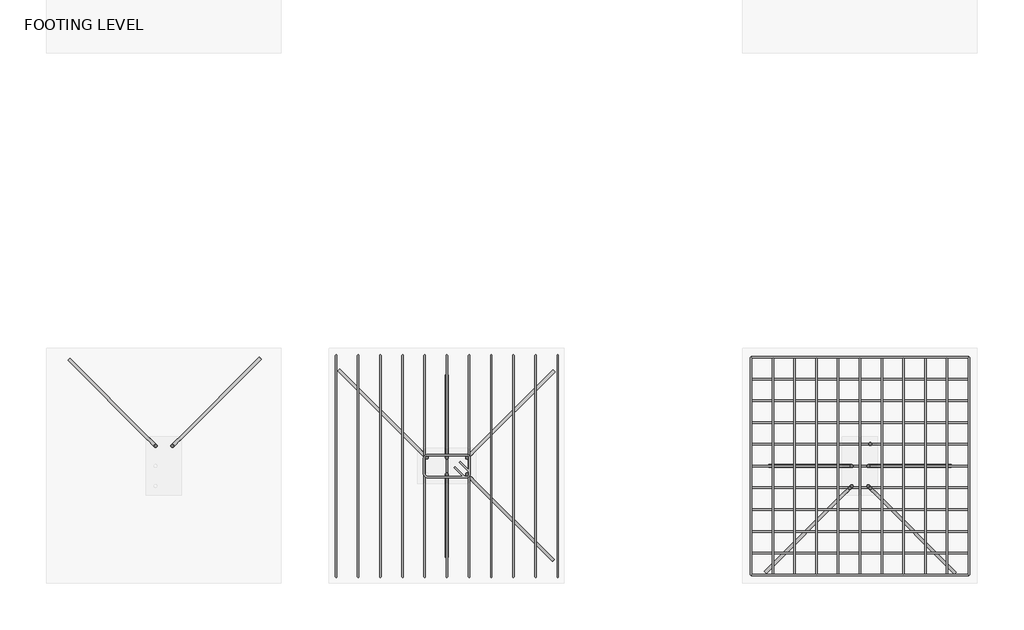
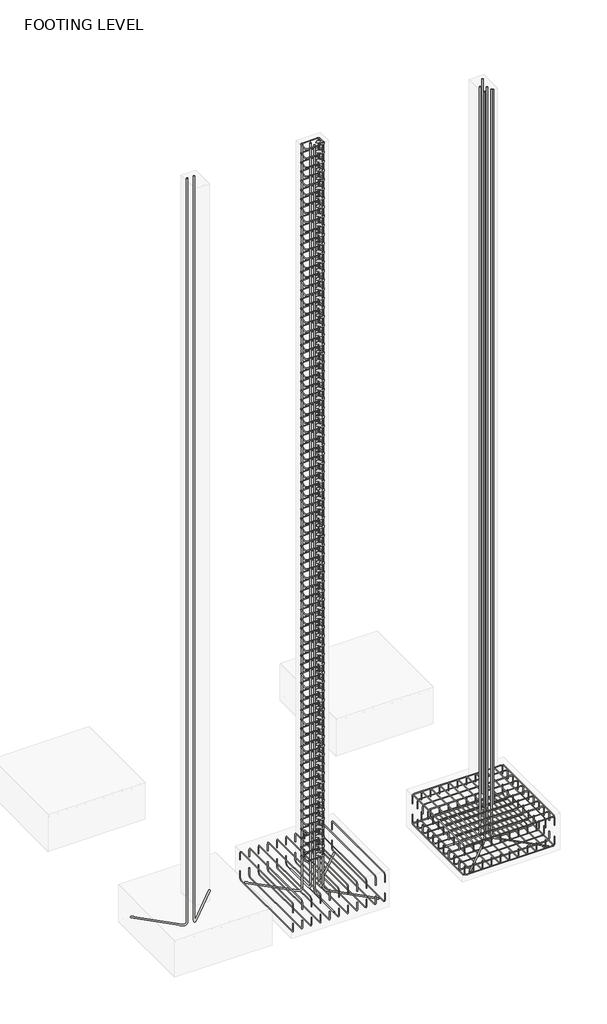
# One storey, part 8 of 10: 23 reinforcing bars.
"""IFC4 building model written with IfcOpenShell, lengths in millimetres."""

from ifc_helpers import new_model, si_unit, point, frame, origin, place, context, project, spatial, polyline, circle_curve, trimmed, segment, composite_curve, source, transform, mapped, element, save
from ifc_brep_helpers import swept_disk

model = new_model("IFC4")

# Units and contexts
model_context = context("Model", 3, world=origin())
ifc_project = project(units=[si_unit("LENGTHUNIT", "METRE", prefix="MILLI")], contexts=[model_context])

# Site, building, storey
site = spatial("IfcSite", under=ifc_project)
building = spatial("IfcBuilding", under=site)
storey = spatial("IfcBuildingStorey", under=building, Name="FOOTING LEVEL", Elevation=-1371.6)

# Reinforcing bars
placement = place(None, origin())
reinforcing_bar_shape = source(origin(), model_context, "Body", "SolidModel", [
    swept_disk(composite_curve([segment(polyline([(-9491.3043223, 10499.0953802, -1574.8), (-9491.3043223, 10499.0953802, -1460.5)]), True, "CONTINUOUS"), segment(trimmed(circle_curve(frame((-9491.3043223, 10465.7578802, -1460.5), z_axis=(1.0, 0.0, 0.0), x_axis=(0.0, 33.337499999999636, 0.0)), 33.3375), [point((-9491.3043223, 10499.0953802, -1460.5))], [point((-9491.3043223, 10465.7578802, -1427.1625))], True, "CARTESIAN"), True, "CONTINUOUS"), segment(polyline([(-9491.3043223, 10465.7578802, -1427.1625), (-9491.3043223, 9119.5578802, -1427.1625)]), True, "CONTINUOUS"), segment(trimmed(circle_curve(frame((-9491.3043223, 9119.5578802, -1460.5), z_axis=(1.0, 0.0, 0.0), x_axis=(0.0, 0.0, 33.33750000000009)), 33.3375), [point((-9491.3043223, 9119.5578802, -1427.1625))], [point((-9491.3043223, 9086.2203802, -1460.5))], True, "CARTESIAN"), True, "CONTINUOUS"), segment(polyline([(-9491.3043223, 9086.2203802, -1460.5), (-9491.3043223, 9086.2203802, -1574.8)]), True, "CONTINUOUS")], self_intersect=False), 4.7625),
])
element("IfcReinforcingBar", 1, at=placement, inside=storey, context=model_context, shape_type="MappedRepresentation", body=[
    mapped(reinforcing_bar_shape, transform((0.0, 0.0, 0.0), x_axis=(1.0, 0.0, 0.0), y_axis=(0.0, 1.0, 0.0), z_axis=(0.0, 0.0, 1.0))),
    mapped(reinforcing_bar_shape, transform((-141.2875, 0.0, 0.0), x_axis=(1.0, 0.0, 0.0), y_axis=(0.0, 1.0, 0.0), z_axis=(0.0, 0.0, 1.0))),
    mapped(reinforcing_bar_shape, transform((-282.575, 0.0, 0.0), x_axis=(1.0, 0.0, 0.0), y_axis=(0.0, 1.0, 0.0), z_axis=(0.0, 0.0, 1.0))),
    mapped(reinforcing_bar_shape, transform((-423.8625, 0.0, 0.0), x_axis=(1.0, 0.0, 0.0), y_axis=(0.0, 1.0, 0.0), z_axis=(0.0, 0.0, 1.0))),
    mapped(reinforcing_bar_shape, transform((-565.15, 0.0, 0.0), x_axis=(1.0, 0.0, 0.0), y_axis=(0.0, 1.0, 0.0), z_axis=(0.0, 0.0, 1.0))),
    mapped(reinforcing_bar_shape, transform((-706.4375, 0.0, 0.0), x_axis=(1.0, 0.0, 0.0), y_axis=(0.0, 1.0, 0.0), z_axis=(0.0, 0.0, 1.0))),
    mapped(reinforcing_bar_shape, transform((-847.725, 0.0, 0.0), x_axis=(1.0, 0.0, 0.0), y_axis=(0.0, 1.0, 0.0), z_axis=(0.0, 0.0, 1.0))),
    mapped(reinforcing_bar_shape, transform((-989.0125, 0.0, 0.0), x_axis=(1.0, 0.0, 0.0), y_axis=(0.0, 1.0, 0.0), z_axis=(0.0, 0.0, 1.0))),
    mapped(reinforcing_bar_shape, transform((-1130.3, 0.0, 0.0), x_axis=(1.0, 0.0, 0.0), y_axis=(0.0, 1.0, 0.0), z_axis=(0.0, 0.0, 1.0))),
    mapped(reinforcing_bar_shape, transform((-1271.5875, 0.0, 0.0), x_axis=(1.0, 0.0, 0.0), y_axis=(0.0, 1.0, 0.0), z_axis=(0.0, 0.0, 1.0))),
    mapped(reinforcing_bar_shape, transform((-1412.875, 0.0, 0.0), x_axis=(1.0, 0.0, 0.0), y_axis=(0.0, 1.0, 0.0), z_axis=(0.0, 0.0, 1.0))),
])
reinforcing_bar_2_shape = source(origin(), model_context, "Body", "SolidModel", [
    swept_disk(composite_curve([segment(polyline([(-9491.3043223, 9086.2203802, -1778.0), (-9491.3043223, 9086.2203802, -1892.3)]), True, "CONTINUOUS"), segment(trimmed(circle_curve(frame((-9491.3043223, 9119.5578802, -1892.3), z_axis=(1.0, 0.0, 0.0), x_axis=(0.0, -33.337499999999636, 0.0)), 33.3375), [point((-9491.3043223, 9086.2203802, -1892.3))], [point((-9491.3043223, 9119.5578802, -1925.6375))], True, "CARTESIAN"), True, "CONTINUOUS"), segment(polyline([(-9491.3043223, 9119.5578802, -1925.6375), (-9491.3043223, 10465.7578802, -1925.6375)]), True, "CONTINUOUS"), segment(trimmed(circle_curve(frame((-9491.3043223, 10465.7578802, -1892.3), z_axis=(1.0, 0.0, 0.0), x_axis=(0.0, 0.0, -33.33750000000009)), 33.3375), [point((-9491.3043223, 10465.7578802, -1925.6375))], [point((-9491.3043223, 10499.0953802, -1892.3))], True, "CARTESIAN"), True, "CONTINUOUS"), segment(polyline([(-9491.3043223, 10499.0953802, -1892.3), (-9491.3043223, 10499.0953802, -1778.0)]), True, "CONTINUOUS")], self_intersect=False), 4.7625),
])
element("IfcReinforcingBar", 2, at=placement, inside=storey, context=model_context, shape_type="MappedRepresentation", body=[
    mapped(reinforcing_bar_2_shape, transform((0.0, 0.0, 0.0), x_axis=(1.0, 0.0, 0.0), y_axis=(0.0, 1.0, 0.0), z_axis=(0.0, 0.0, 1.0))),
    mapped(reinforcing_bar_2_shape, transform((-141.2875, 0.0, 0.0), x_axis=(1.0, 0.0, 0.0), y_axis=(0.0, 1.0, 0.0), z_axis=(0.0, 0.0, 1.0))),
    mapped(reinforcing_bar_2_shape, transform((-282.575, 0.0, 0.0), x_axis=(1.0, 0.0, 0.0), y_axis=(0.0, 1.0, 0.0), z_axis=(0.0, 0.0, 1.0))),
    mapped(reinforcing_bar_2_shape, transform((-423.8625, 0.0, 0.0), x_axis=(1.0, 0.0, 0.0), y_axis=(0.0, 1.0, 0.0), z_axis=(0.0, 0.0, 1.0))),
    mapped(reinforcing_bar_2_shape, transform((-565.15, 0.0, 0.0), x_axis=(1.0, 0.0, 0.0), y_axis=(0.0, 1.0, 0.0), z_axis=(0.0, 0.0, 1.0))),
    mapped(reinforcing_bar_2_shape, transform((-706.4375, 0.0, 0.0), x_axis=(1.0, 0.0, 0.0), y_axis=(0.0, 1.0, 0.0), z_axis=(0.0, 0.0, 1.0))),
    mapped(reinforcing_bar_2_shape, transform((-847.725, 0.0, 0.0), x_axis=(1.0, 0.0, 0.0), y_axis=(0.0, 1.0, 0.0), z_axis=(0.0, 0.0, 1.0))),
    mapped(reinforcing_bar_2_shape, transform((-989.0125, 0.0, 0.0), x_axis=(1.0, 0.0, 0.0), y_axis=(0.0, 1.0, 0.0), z_axis=(0.0, 0.0, 1.0))),
    mapped(reinforcing_bar_2_shape, transform((-1130.3, 0.0, 0.0), x_axis=(1.0, 0.0, 0.0), y_axis=(0.0, 1.0, 0.0), z_axis=(0.0, 0.0, 1.0))),
    mapped(reinforcing_bar_2_shape, transform((-1271.5875, 0.0, 0.0), x_axis=(1.0, 0.0, 0.0), y_axis=(0.0, 1.0, 0.0), z_axis=(0.0, 0.0, 1.0))),
    mapped(reinforcing_bar_2_shape, transform((-1412.875, 0.0, 0.0), x_axis=(1.0, 0.0, 0.0), y_axis=(0.0, 1.0, 0.0), z_axis=(0.0, 0.0, 1.0))),
])
reinforcing_bar_3_shape = source(origin(), model_context, "Body", "SolidModel", [
    swept_disk(composite_curve([segment(polyline([(-10904.1793223, 9086.2203802, -1770.864029), (-10904.1793223, 9086.2203802, -1885.164029)]), True, "CONTINUOUS"), segment(trimmed(circle_curve(frame((-10870.8418223, 9086.2203802, -1885.164029), z_axis=(0.0, -1.0, 0.0), x_axis=(-33.337499999999636, 0.0, 0.0)), 33.3375), [point((-10904.1793223, 9086.2203802, -1885.164029))], [point((-10870.8418223, 9086.2203802, -1918.501529))], True, "CARTESIAN"), True, "CONTINUOUS"), segment(polyline([(-10870.8418223, 9086.2203802, -1918.501529), (-9524.6418223, 9086.2203802, -1918.501529)]), True, "CONTINUOUS"), segment(trimmed(circle_curve(frame((-9524.6418223, 9086.2203802, -1885.164029), z_axis=(0.0, -1.0, 0.0), x_axis=(0.0, 0.0, -33.337499999999864)), 33.3375), [point((-9524.6418223, 9086.2203802, -1918.501529))], [point((-9491.3043223, 9086.2203802, -1885.164029))], True, "CARTESIAN"), True, "CONTINUOUS"), segment(polyline([(-9491.3043223, 9086.2203802, -1885.164029), (-9491.3043223, 9086.2203802, -1770.864029)]), True, "CONTINUOUS")], self_intersect=False), 4.7625),
])
element("IfcReinforcingBar", 3, at=placement, inside=storey, context=model_context, shape_type="MappedRepresentation", body=[
    mapped(reinforcing_bar_3_shape, transform((0.0, 0.0, 0.0), x_axis=(1.0, 0.0, 0.0), y_axis=(0.0, 1.0, 0.0), z_axis=(0.0, 0.0, 1.0))),
    mapped(reinforcing_bar_3_shape, transform((0.0, 141.2875, 0.0), x_axis=(1.0, 0.0, 0.0), y_axis=(0.0, 1.0, 0.0), z_axis=(0.0, 0.0, 1.0))),
    mapped(reinforcing_bar_3_shape, transform((0.0, 282.575, 0.0), x_axis=(1.0, 0.0, 0.0), y_axis=(0.0, 1.0, 0.0), z_axis=(0.0, 0.0, 1.0))),
    mapped(reinforcing_bar_3_shape, transform((0.0, 423.8625, 0.0), x_axis=(1.0, 0.0, 0.0), y_axis=(0.0, 1.0, 0.0), z_axis=(0.0, 0.0, 1.0))),
    mapped(reinforcing_bar_3_shape, transform((0.0, 565.15, 0.0), x_axis=(1.0, 0.0, 0.0), y_axis=(0.0, 1.0, 0.0), z_axis=(0.0, 0.0, 1.0))),
    mapped(reinforcing_bar_3_shape, transform((0.0, 706.4375, 0.0), x_axis=(1.0, 0.0, 0.0), y_axis=(0.0, 1.0, 0.0), z_axis=(0.0, 0.0, 1.0))),
    mapped(reinforcing_bar_3_shape, transform((0.0, 847.725, 0.0), x_axis=(1.0, 0.0, 0.0), y_axis=(0.0, 1.0, 0.0), z_axis=(0.0, 0.0, 1.0))),
    mapped(reinforcing_bar_3_shape, transform((0.0, 989.0125, 0.0), x_axis=(1.0, 0.0, 0.0), y_axis=(0.0, 1.0, 0.0), z_axis=(0.0, 0.0, 1.0))),
    mapped(reinforcing_bar_3_shape, transform((0.0, 1130.3, 0.0), x_axis=(1.0, 0.0, 0.0), y_axis=(0.0, 1.0, 0.0), z_axis=(0.0, 0.0, 1.0))),
    mapped(reinforcing_bar_3_shape, transform((0.0, 1271.5875, 0.0), x_axis=(1.0, 0.0, 0.0), y_axis=(0.0, 1.0, 0.0), z_axis=(0.0, 0.0, 1.0))),
    mapped(reinforcing_bar_3_shape, transform((0.0, 1412.875, 0.0), x_axis=(1.0, 0.0, 0.0), y_axis=(0.0, 1.0, 0.0), z_axis=(0.0, 0.0, 1.0))),
])
reinforcing_bar_4_shape = source(origin(), model_context, "Body", "SolidModel", [
    swept_disk(composite_curve([segment(polyline([(-10904.1793223, 10499.0953802, -1586.5406765), (-10904.1793223, 10499.0953802, -1472.2406765)]), True, "CONTINUOUS"), segment(trimmed(circle_curve(frame((-10870.8418223, 10499.0953802, -1472.2406765), z_axis=(0.0, 1.0, 0.0), x_axis=(-33.337499999999636, 0.0, 0.0)), 33.3375), [point((-10904.1793223, 10499.0953802, -1472.2406765))], [point((-10870.8418223, 10499.0953802, -1438.9031765))], True, "CARTESIAN"), True, "CONTINUOUS"), segment(polyline([(-10870.8418223, 10499.0953802, -1438.9031765), (-9524.6418223, 10499.0953802, -1438.9031765)]), True, "CONTINUOUS"), segment(trimmed(circle_curve(frame((-9524.6418223, 10499.0953802, -1472.2406765), z_axis=(0.0, 1.0, 0.0), x_axis=(0.0, 0.0, 33.33750000000009)), 33.3375), [point((-9524.6418223, 10499.0953802, -1438.9031765))], [point((-9491.3043223, 10499.0953802, -1472.2406765))], True, "CARTESIAN"), True, "CONTINUOUS"), segment(polyline([(-9491.3043223, 10499.0953802, -1472.2406765), (-9491.3043223, 10499.0953802, -1586.5406765)]), True, "CONTINUOUS")], self_intersect=False), 4.7625),
])
element("IfcReinforcingBar", 4, at=placement, inside=storey, context=model_context, shape_type="MappedRepresentation", body=[
    mapped(reinforcing_bar_4_shape, transform((0.0, 0.0, 0.0), x_axis=(1.0, 0.0, 0.0), y_axis=(0.0, 1.0, 0.0), z_axis=(0.0, 0.0, 1.0))),
    mapped(reinforcing_bar_4_shape, transform((0.0, -141.2875, 0.0), x_axis=(1.0, 0.0, 0.0), y_axis=(0.0, 1.0, 0.0), z_axis=(0.0, 0.0, 1.0))),
    mapped(reinforcing_bar_4_shape, transform((0.0, -282.575, 0.0), x_axis=(1.0, 0.0, 0.0), y_axis=(0.0, 1.0, 0.0), z_axis=(0.0, 0.0, 1.0))),
    mapped(reinforcing_bar_4_shape, transform((0.0, -423.8625, 0.0), x_axis=(1.0, 0.0, 0.0), y_axis=(0.0, 1.0, 0.0), z_axis=(0.0, 0.0, 1.0))),
    mapped(reinforcing_bar_4_shape, transform((0.0, -565.15, 0.0), x_axis=(1.0, 0.0, 0.0), y_axis=(0.0, 1.0, 0.0), z_axis=(0.0, 0.0, 1.0))),
    mapped(reinforcing_bar_4_shape, transform((0.0, -706.4375, 0.0), x_axis=(1.0, 0.0, 0.0), y_axis=(0.0, 1.0, 0.0), z_axis=(0.0, 0.0, 1.0))),
    mapped(reinforcing_bar_4_shape, transform((0.0, -847.725, 0.0), x_axis=(1.0, 0.0, 0.0), y_axis=(0.0, 1.0, 0.0), z_axis=(0.0, 0.0, 1.0))),
    mapped(reinforcing_bar_4_shape, transform((0.0, -989.0125, 0.0), x_axis=(1.0, 0.0, 0.0), y_axis=(0.0, 1.0, 0.0), z_axis=(0.0, 0.0, 1.0))),
    mapped(reinforcing_bar_4_shape, transform((0.0, -1130.3, 0.0), x_axis=(1.0, 0.0, 0.0), y_axis=(0.0, 1.0, 0.0), z_axis=(0.0, 0.0, 1.0))),
    mapped(reinforcing_bar_4_shape, transform((0.0, -1271.5875, 0.0), x_axis=(1.0, 0.0, 0.0), y_axis=(0.0, 1.0, 0.0), z_axis=(0.0, 0.0, 1.0))),
    mapped(reinforcing_bar_4_shape, transform((0.0, -1412.875, 0.0), x_axis=(1.0, 0.0, 0.0), y_axis=(0.0, 1.0, 0.0), z_axis=(0.0, 0.0, 1.0))),
])
reinforcing_bar_5_shape = source(origin(), model_context, "Body", "SolidModel", [
    swept_disk(composite_curve([segment(polyline([(-12158.3043223, 9073.5203802, -1770.864029), (-12158.3043223, 9073.5203802, -1885.164029)]), True, "CONTINUOUS"), segment(trimmed(circle_curve(frame((-12158.3043223, 9106.8578802, -1885.164029), z_axis=(1.0, 0.0, 0.0), x_axis=(0.0, -33.337499999999636, 0.0)), 33.3375), [point((-12158.3043223, 9073.5203802, -1885.164029))], [point((-12158.3043223, 9106.8578802, -1918.501529))], True, "CARTESIAN"), True, "CONTINUOUS"), segment(polyline([(-12158.3043223, 9106.8578802, -1918.501529), (-12158.3043223, 10478.4578802, -1918.501529)]), True, "CONTINUOUS"), segment(trimmed(circle_curve(frame((-12158.3043223, 10478.4578802, -1885.164029), z_axis=(1.0, 0.0, 0.0), x_axis=(0.0, 0.0, -33.337499999999864)), 33.3375), [point((-12158.3043223, 10478.4578802, -1918.501529))], [point((-12158.3043223, 10511.7953802, -1885.164029))], True, "CARTESIAN"), True, "CONTINUOUS"), segment(polyline([(-12158.3043223, 10511.7953802, -1885.164029), (-12158.3043223, 10511.7953802, -1770.864029)]), True, "CONTINUOUS")], self_intersect=False), 4.7625),
])
element("IfcReinforcingBar", 5, at=placement, inside=storey, context=model_context, shape_type="MappedRepresentation", body=[
    mapped(reinforcing_bar_5_shape, transform((0.0, 0.0, 0.0), x_axis=(1.0, 0.0, 0.0), y_axis=(0.0, 1.0, 0.0), z_axis=(0.0, 0.0, 1.0))),
    mapped(reinforcing_bar_5_shape, transform((-143.8275, 0.0, 0.0), x_axis=(1.0, 0.0, 0.0), y_axis=(0.0, 1.0, 0.0), z_axis=(0.0, 0.0, 1.0))),
    mapped(reinforcing_bar_5_shape, transform((-287.655, 0.0, 0.0), x_axis=(1.0, 0.0, 0.0), y_axis=(0.0, 1.0, 0.0), z_axis=(0.0, 0.0, 1.0))),
    mapped(reinforcing_bar_5_shape, transform((-431.4825, 0.0, 0.0), x_axis=(1.0, 0.0, 0.0), y_axis=(0.0, 1.0, 0.0), z_axis=(0.0, 0.0, 1.0))),
    mapped(reinforcing_bar_5_shape, transform((-575.31, 0.0, 0.0), x_axis=(1.0, 0.0, 0.0), y_axis=(0.0, 1.0, 0.0), z_axis=(0.0, 0.0, 1.0))),
    mapped(reinforcing_bar_5_shape, transform((-719.1375, 0.0, 0.0), x_axis=(1.0, 0.0, 0.0), y_axis=(0.0, 1.0, 0.0), z_axis=(0.0, 0.0, 1.0))),
    mapped(reinforcing_bar_5_shape, transform((-862.965, 0.0, 0.0), x_axis=(1.0, 0.0, 0.0), y_axis=(0.0, 1.0, 0.0), z_axis=(0.0, 0.0, 1.0))),
    mapped(reinforcing_bar_5_shape, transform((-1006.7925, 0.0, 0.0), x_axis=(1.0, 0.0, 0.0), y_axis=(0.0, 1.0, 0.0), z_axis=(0.0, 0.0, 1.0))),
    mapped(reinforcing_bar_5_shape, transform((-1150.62, 0.0, 0.0), x_axis=(1.0, 0.0, 0.0), y_axis=(0.0, 1.0, 0.0), z_axis=(0.0, 0.0, 1.0))),
    mapped(reinforcing_bar_5_shape, transform((-1294.4475, 0.0, 0.0), x_axis=(1.0, 0.0, 0.0), y_axis=(0.0, 1.0, 0.0), z_axis=(0.0, 0.0, 1.0))),
    mapped(reinforcing_bar_5_shape, transform((-1438.275, 0.0, 0.0), x_axis=(1.0, 0.0, 0.0), y_axis=(0.0, 1.0, 0.0), z_axis=(0.0, 0.0, 1.0))),
])
reinforcing_bar_6_shape = source(origin(), model_context, "Body", "SolidModel", [
    swept_disk(composite_curve([segment(polyline([(-13596.5793223, 9073.5203802, -1586.5406765), (-13596.5793223, 9073.5203802, -1472.2406765)]), True, "CONTINUOUS"), segment(trimmed(circle_curve(frame((-13596.5793223, 9106.8578802, -1472.2406765), z_axis=(-1.0, 0.0, 0.0), x_axis=(0.0, -33.337499999999636, 0.0)), 33.3375), [point((-13596.5793223, 9073.5203802, -1472.2406765))], [point((-13596.5793223, 9106.8578802, -1438.9031765))], True, "CARTESIAN"), True, "CONTINUOUS"), segment(polyline([(-13596.5793223, 9106.8578802, -1438.9031765), (-13596.5793223, 10478.4578802, -1438.9031765)]), True, "CONTINUOUS"), segment(trimmed(circle_curve(frame((-13596.5793223, 10478.4578802, -1472.2406765), z_axis=(-1.0, 0.0, 0.0), x_axis=(0.0, 0.0, 33.33750000000009)), 33.3375), [point((-13596.5793223, 10478.4578802, -1438.9031765))], [point((-13596.5793223, 10511.7953802, -1472.2406765))], True, "CARTESIAN"), True, "CONTINUOUS"), segment(polyline([(-13596.5793223, 10511.7953802, -1472.2406765), (-13596.5793223, 10511.7953802, -1586.5406765)]), True, "CONTINUOUS")], self_intersect=False), 4.7625),
])
element("IfcReinforcingBar", 6, at=placement, inside=storey, context=model_context, shape_type="MappedRepresentation", body=[
    mapped(reinforcing_bar_6_shape, transform((0.0, 0.0, 0.0), x_axis=(1.0, 0.0, 0.0), y_axis=(0.0, 1.0, 0.0), z_axis=(0.0, 0.0, 1.0))),
    mapped(reinforcing_bar_6_shape, transform((143.8275, 0.0, 0.0), x_axis=(1.0, 0.0, 0.0), y_axis=(0.0, 1.0, 0.0), z_axis=(0.0, 0.0, 1.0))),
    mapped(reinforcing_bar_6_shape, transform((287.655, 0.0, 0.0), x_axis=(1.0, 0.0, 0.0), y_axis=(0.0, 1.0, 0.0), z_axis=(0.0, 0.0, 1.0))),
    mapped(reinforcing_bar_6_shape, transform((431.4825, 0.0, 0.0), x_axis=(1.0, 0.0, 0.0), y_axis=(0.0, 1.0, 0.0), z_axis=(0.0, 0.0, 1.0))),
    mapped(reinforcing_bar_6_shape, transform((575.31, 0.0, 0.0), x_axis=(1.0, 0.0, 0.0), y_axis=(0.0, 1.0, 0.0), z_axis=(0.0, 0.0, 1.0))),
    mapped(reinforcing_bar_6_shape, transform((719.1375, 0.0, 0.0), x_axis=(1.0, 0.0, 0.0), y_axis=(0.0, 1.0, 0.0), z_axis=(0.0, 0.0, 1.0))),
    mapped(reinforcing_bar_6_shape, transform((862.965, 0.0, 0.0), x_axis=(1.0, 0.0, 0.0), y_axis=(0.0, 1.0, 0.0), z_axis=(0.0, 0.0, 1.0))),
    mapped(reinforcing_bar_6_shape, transform((1006.7925, 0.0, 0.0), x_axis=(1.0, 0.0, 0.0), y_axis=(0.0, 1.0, 0.0), z_axis=(0.0, 0.0, 1.0))),
    mapped(reinforcing_bar_6_shape, transform((1150.62, 0.0, 0.0), x_axis=(1.0, 0.0, 0.0), y_axis=(0.0, 1.0, 0.0), z_axis=(0.0, 0.0, 1.0))),
    mapped(reinforcing_bar_6_shape, transform((1294.4475, 0.0, 0.0), x_axis=(1.0, 0.0, 0.0), y_axis=(0.0, 1.0, 0.0), z_axis=(0.0, 0.0, 1.0))),
    mapped(reinforcing_bar_6_shape, transform((1438.275, 0.0, 0.0), x_axis=(1.0, 0.0, 0.0), y_axis=(0.0, 1.0, 0.0), z_axis=(0.0, 0.0, 1.0))),
])
element("IfcReinforcingBar", 7, at=placement, inside=storey, context=model_context, shape_type="SolidModel", body=[
    swept_disk(composite_curve([segment(polyline([(-15328.6277703, 10484.8938282, -1910.4342608), (-14814.0983591, 9970.3644169, -1910.4342608)]), True, "CONTINUOUS"), segment(trimmed(circle_curve(frame((-14814.0983591, 9970.3644169, -1843.7592608), z_axis=(-0.7071067811865736, -0.7071067811865216, 0.0), x_axis=(0.0, 0.0, -66.67499999999995)), 66.675), [point((-14814.0983591, 9970.3644169, -1910.4342608))], [point((-14766.9520144, 9923.2180723, -1843.7592608))], True, "CARTESIAN"), True, "CONTINUOUS"), segment(polyline([(-14766.9520144, 9923.2180723, -1843.7592608), (-14766.9520144, 9923.2180723, 10477.5)]), True, "CONTINUOUS")], self_intersect=False), 9.525),
])
element("IfcReinforcingBar", 8, at=placement, inside=storey, context=model_context, shape_type="SolidModel", body=[
    swept_disk(composite_curve([segment(polyline([(-14088.5374965, 10492.912206, -1910.4342608), (-14611.0852856, 9970.3644169, -1910.4342608)]), True, "CONTINUOUS"), segment(trimmed(circle_curve(frame((-14611.0852856, 9970.3644169, -1843.7592608), z_axis=(-0.7071067811865712, 0.7071067811865238, 0.0), x_axis=(0.0, 0.0, -66.67499999999995)), 66.675), [point((-14611.0852856, 9970.3644169, -1910.4342608))], [point((-14658.2316302, 9923.2180723, -1843.7592608))], True, "CARTESIAN"), True, "CONTINUOUS"), segment(polyline([(-14658.2316302, 9923.2180723, -1843.7592608), (-14658.2316302, 9923.2180723, 10477.5)]), True, "CONTINUOUS")], self_intersect=False), 9.525),
])
element("IfcReinforcingBar", 9, at=placement, inside=storey, context=model_context, shape_type="SolidModel", body=[
    swept_disk(composite_curve([segment(polyline([(-10130.6816302, 9935.9180723, -1346.2), (-10130.6816302, 9935.9180723, 10490.2)]), True, "CONTINUOUS")], self_intersect=False), 9.525),
])
element("IfcReinforcingBar", 10, at=placement, inside=storey, context=model_context, shape_type="SolidModel", body=[
    swept_disk(composite_curve([segment(polyline([(-10264.8020144, 9649.3976881, -1346.2), (-10264.8020144, 9649.3976881, 10490.2)]), True, "CONTINUOUS")], self_intersect=False), 9.525),
])
element("IfcReinforcingBar", 11, at=placement, inside=storey, context=model_context, shape_type="SolidModel", body=[
    swept_disk(composite_curve([segment(polyline([(-10130.6816302, 9649.3976881, -1346.2), (-10130.6816302, 9649.3976881, 10490.2)]), True, "CONTINUOUS")], self_intersect=False), 9.525),
])
element("IfcReinforcingBar", 12, at=placement, inside=storey, context=model_context, shape_type="SolidModel", body=[
    swept_disk(composite_curve([segment(polyline([(-10810.8211349, 9103.3785676, -1910.4342608), (-10299.2483591, 9614.9513434, -1910.4342608)]), True, "CONTINUOUS"), segment(trimmed(circle_curve(frame((-10299.2483591, 9614.9513434, -1843.7592608), z_axis=(0.7071067811865759, -0.7071067811865193, 0.0), x_axis=(0.0, 0.0, -66.67499999999995)), 66.675), [point((-10299.2483591, 9614.9513434, -1910.4342608))], [point((-10252.1020144, 9662.0976881, -1843.7592608))], True, "CARTESIAN"), True, "CONTINUOUS"), segment(polyline([(-10252.1020144, 9662.0976881, -1843.7592608), (-10252.1020144, 9662.0976881, 10490.2)]), True, "CONTINUOUS")], self_intersect=False), 9.525),
])
element("IfcReinforcingBar", 13, at=placement, inside=storey, context=model_context, shape_type="SolidModel", body=[
    swept_disk(composite_curve([segment(polyline([(-9579.2028099, 9097.9188678, -1910.4342608), (-10096.2352856, 9614.9513434, -1910.4342608)]), True, "CONTINUOUS"), segment(trimmed(circle_curve(frame((-10096.2352856, 9614.9513434, -1843.7592608), z_axis=(0.707106781186569, 0.707106781186526, 0.0), x_axis=(0.0, 0.0, -66.67499999999995)), 66.675), [point((-10096.2352856, 9614.9513434, -1910.4342608))], [point((-10143.3816302, 9662.0976881, -1843.7592608))], True, "CARTESIAN"), True, "CONTINUOUS"), segment(polyline([(-10143.3816302, 9662.0976881, -1843.7592608), (-10143.3816302, 9662.0976881, 10490.2)]), True, "CONTINUOUS")], self_intersect=False), 9.525),
])
element("IfcReinforcingBar", 14, at=placement, inside=storey, context=model_context, shape_type="SolidModel", body=[
    swept_disk(composite_curve([segment(polyline([(-10790.3318909, 9792.6578802, -1910.4342608), (-10318.7770144, 9792.6578802, -1910.4342608)]), True, "CONTINUOUS"), segment(trimmed(circle_curve(frame((-10318.7770144, 9792.6578802, -1843.7592608), z_axis=(0.0, -1.0, 0.0), x_axis=(0.0, 0.0, -66.67499999999995)), 66.675), [point((-10318.7770144, 9792.6578802, -1910.4342608))], [point((-10252.1020144, 9792.6578802, -1843.7592608))], True, "CARTESIAN"), True, "CONTINUOUS"), segment(polyline([(-10252.1020144, 9792.6578802, -1843.7592608), (-10252.1020144, 9792.6578802, 10490.2)]), True, "CONTINUOUS")], self_intersect=False), 9.525),
])
element("IfcReinforcingBar", 15, at=placement, inside=storey, context=model_context, shape_type="SolidModel", body=[
    swept_disk(composite_curve([segment(polyline([(-9605.1517538, 9792.6578802, -1916.7848067), (-10076.7066302, 9792.6578802, -1916.7848067)]), True, "CONTINUOUS"), segment(trimmed(circle_curve(frame((-10076.7066302, 9792.6578802, -1850.1098067), z_axis=(0.0, 1.0, 0.0), x_axis=(0.0, 0.0, -66.67499999999995)), 66.675), [point((-10076.7066302, 9792.6578802, -1916.7848067))], [point((-10143.3816302, 9792.6578802, -1850.1098067))], True, "CARTESIAN"), True, "CONTINUOUS"), segment(polyline([(-10143.3816302, 9792.6578802, -1850.1098067), (-10143.3816302, 9792.6578802, 10449.7223493)]), True, "CONTINUOUS")], self_intersect=False), 9.525),
])
reinforcing_bar_7_shape = source(origin(), model_context, "Body", "SolidModel", [
    swept_disk(composite_curve([segment(polyline([(-12827.3189996, 9785.059097, -1328.7375), (-12770.4548026, 9728.1948999, -1328.7375)]), True, "CONTINUOUS"), segment(trimmed(circle_curve(frame((-12753.6168223, 9745.0328802, -1328.7375), z_axis=(0.0, 0.0, 1.0), x_axis=(-16.83798029999889, -16.83798030000071, 0.0)), 23.8125), [point((-12770.4548026, 9728.1948999, -1328.7375))], [point((-12729.8043223, 9745.0328802, -1328.7375))], True, "CARTESIAN"), True, "CONTINUOUS"), segment(polyline([(-12729.8043223, 9745.0328802, -1328.7375), (-12729.8043223, 9840.2828802, -1328.7375)]), True, "CONTINUOUS"), segment(trimmed(circle_curve(frame((-12753.6168223, 9840.2828802, -1328.7375), z_axis=(0.0, 0.0, 1.0), x_axis=(23.8125, 0.0, 0.0)), 23.8125), [point((-12729.8043223, 9840.2828802, -1328.7375))], [point((-12753.6168223, 9864.0953802, -1328.7375))], True, "CARTESIAN"), True, "CONTINUOUS"), segment(polyline([(-12753.6168223, 9864.0953802, -1328.7375), (-13001.2668223, 9864.0953802, -1328.7375)]), True, "CONTINUOUS"), segment(trimmed(circle_curve(frame((-13001.2668223, 9840.3356211, -1330.3214839), z_axis=(0.0, -0.06651901052377396, 0.9977851578566089), x_axis=(0.0, 23.759759100001247, 1.583983900000021)), 23.8125), [point((-13001.2668223, 9864.0953802, -1328.7375))], [point((-13025.0793223, 9840.3356211, -1330.3214839))], True, "CARTESIAN"), True, "CONTINUOUS"), segment(polyline([(-13025.0793223, 9840.3356211, -1330.3214839), (-13025.0793223, 9744.9801392, -1336.6785161)]), True, "CONTINUOUS"), segment(trimmed(circle_curve(frame((-13001.2668223, 9744.9801392, -1336.6785161), z_axis=(0.0, -0.06651901052377396, 0.9977851578566089), x_axis=(-23.8125, 0.0, 0.0)), 23.8125), [point((-13025.0793223, 9744.9801392, -1336.6785161))], [point((-13001.2668223, 9721.2203802, -1338.2625))], True, "CARTESIAN"), True, "CONTINUOUS"), segment(polyline([(-13001.2668223, 9721.2203802, -1338.2625), (-12753.6168223, 9721.2203802, -1338.2625)]), True, "CONTINUOUS"), segment(trimmed(circle_curve(frame((-12753.6168223, 9745.0328802, -1338.2625), z_axis=(0.0, 0.0, 1.0), x_axis=(0.0, -23.8125, 0.0)), 23.8125), [point((-12753.6168223, 9721.2203802, -1338.2625))], [point((-12736.7788421, 9761.8708604, -1338.2625))], True, "CARTESIAN"), True, "CONTINUOUS"), segment(polyline([(-12736.7788421, 9761.8708604, -1338.2625), (-12793.6430392, 9818.7350575, -1338.2625)]), True, "CONTINUOUS")], self_intersect=False), 4.7625),
])
element("IfcReinforcingBar", 16, at=placement, inside=storey, context=model_context, shape_type="MappedRepresentation", body=[
    mapped(reinforcing_bar_7_shape, transform((0.0, 0.0, 0.0), x_axis=(1.0, 0.0, 0.0), y_axis=(0.0, 1.0, 0.0), z_axis=(0.0, 0.0, 1.0))),
    mapped(reinforcing_bar_7_shape, transform((0.0, 0.0, 151.3009615), x_axis=(1.0, 0.0, 0.0), y_axis=(0.0, 1.0, 0.0), z_axis=(0.0, 0.0, 1.0))),
    mapped(reinforcing_bar_7_shape, transform((0.0, 0.0, 302.6019231), x_axis=(1.0, 0.0, 0.0), y_axis=(0.0, 1.0, 0.0), z_axis=(0.0, 0.0, 1.0))),
    mapped(reinforcing_bar_7_shape, transform((0.0, 0.0, 453.9028846), x_axis=(1.0, 0.0, 0.0), y_axis=(0.0, 1.0, 0.0), z_axis=(0.0, 0.0, 1.0))),
    mapped(reinforcing_bar_7_shape, transform((0.0, 0.0, 605.2038462), x_axis=(1.0, 0.0, 0.0), y_axis=(0.0, 1.0, 0.0), z_axis=(0.0, 0.0, 1.0))),
    mapped(reinforcing_bar_7_shape, transform((0.0, 0.0, 756.5048077), x_axis=(1.0, 0.0, 0.0), y_axis=(0.0, 1.0, 0.0), z_axis=(0.0, 0.0, 1.0))),
    mapped(reinforcing_bar_7_shape, transform((0.0, 0.0, 907.8057692), x_axis=(1.0, 0.0, 0.0), y_axis=(0.0, 1.0, 0.0), z_axis=(0.0, 0.0, 1.0))),
    mapped(reinforcing_bar_7_shape, transform((0.0, 0.0, 1059.1067308), x_axis=(1.0, 0.0, 0.0), y_axis=(0.0, 1.0, 0.0), z_axis=(0.0, 0.0, 1.0))),
    mapped(reinforcing_bar_7_shape, transform((0.0, 0.0, 1210.4076923), x_axis=(1.0, 0.0, 0.0), y_axis=(0.0, 1.0, 0.0), z_axis=(0.0, 0.0, 1.0))),
    mapped(reinforcing_bar_7_shape, transform((0.0, 0.0, 1361.7086538), x_axis=(1.0, 0.0, 0.0), y_axis=(0.0, 1.0, 0.0), z_axis=(0.0, 0.0, 1.0))),
    mapped(reinforcing_bar_7_shape, transform((0.0, 0.0, 1513.0096154), x_axis=(1.0, 0.0, 0.0), y_axis=(0.0, 1.0, 0.0), z_axis=(0.0, 0.0, 1.0))),
    mapped(reinforcing_bar_7_shape, transform((0.0, 0.0, 1664.3105769), x_axis=(1.0, 0.0, 0.0), y_axis=(0.0, 1.0, 0.0), z_axis=(0.0, 0.0, 1.0))),
    mapped(reinforcing_bar_7_shape, transform((0.0, 0.0, 1815.6115385), x_axis=(1.0, 0.0, 0.0), y_axis=(0.0, 1.0, 0.0), z_axis=(0.0, 0.0, 1.0))),
    mapped(reinforcing_bar_7_shape, transform((0.0, 0.0, 1966.9125), x_axis=(1.0, 0.0, 0.0), y_axis=(0.0, 1.0, 0.0), z_axis=(0.0, 0.0, 1.0))),
    mapped(reinforcing_bar_7_shape, transform((0.0, 0.0, 2118.2134615), x_axis=(1.0, 0.0, 0.0), y_axis=(0.0, 1.0, 0.0), z_axis=(0.0, 0.0, 1.0))),
    mapped(reinforcing_bar_7_shape, transform((0.0, 0.0, 2269.5144231), x_axis=(1.0, 0.0, 0.0), y_axis=(0.0, 1.0, 0.0), z_axis=(0.0, 0.0, 1.0))),
    mapped(reinforcing_bar_7_shape, transform((0.0, 0.0, 2420.8153846), x_axis=(1.0, 0.0, 0.0), y_axis=(0.0, 1.0, 0.0), z_axis=(0.0, 0.0, 1.0))),
    mapped(reinforcing_bar_7_shape, transform((0.0, 0.0, 2572.1163462), x_axis=(1.0, 0.0, 0.0), y_axis=(0.0, 1.0, 0.0), z_axis=(0.0, 0.0, 1.0))),
    mapped(reinforcing_bar_7_shape, transform((0.0, 0.0, 2723.4173077), x_axis=(1.0, 0.0, 0.0), y_axis=(0.0, 1.0, 0.0), z_axis=(0.0, 0.0, 1.0))),
    mapped(reinforcing_bar_7_shape, transform((0.0, 0.0, 2874.7182692), x_axis=(1.0, 0.0, 0.0), y_axis=(0.0, 1.0, 0.0), z_axis=(0.0, 0.0, 1.0))),
    mapped(reinforcing_bar_7_shape, transform((0.0, 0.0, 3026.0192308), x_axis=(1.0, 0.0, 0.0), y_axis=(0.0, 1.0, 0.0), z_axis=(0.0, 0.0, 1.0))),
    mapped(reinforcing_bar_7_shape, transform((0.0, 0.0, 3177.3201923), x_axis=(1.0, 0.0, 0.0), y_axis=(0.0, 1.0, 0.0), z_axis=(0.0, 0.0, 1.0))),
    mapped(reinforcing_bar_7_shape, transform((0.0, 0.0, 3328.6211538), x_axis=(1.0, 0.0, 0.0), y_axis=(0.0, 1.0, 0.0), z_axis=(0.0, 0.0, 1.0))),
    mapped(reinforcing_bar_7_shape, transform((0.0, 0.0, 3479.9221154), x_axis=(1.0, 0.0, 0.0), y_axis=(0.0, 1.0, 0.0), z_axis=(0.0, 0.0, 1.0))),
    mapped(reinforcing_bar_7_shape, transform((0.0, 0.0, 3631.2230769), x_axis=(1.0, 0.0, 0.0), y_axis=(0.0, 1.0, 0.0), z_axis=(0.0, 0.0, 1.0))),
    mapped(reinforcing_bar_7_shape, transform((0.0, 0.0, 3782.5240385), x_axis=(1.0, 0.0, 0.0), y_axis=(0.0, 1.0, 0.0), z_axis=(0.0, 0.0, 1.0))),
    mapped(reinforcing_bar_7_shape, transform((0.0, 0.0, 3933.825), x_axis=(1.0, 0.0, 0.0), y_axis=(0.0, 1.0, 0.0), z_axis=(0.0, 0.0, 1.0))),
    mapped(reinforcing_bar_7_shape, transform((0.0, 0.0, 4085.1259615), x_axis=(1.0, 0.0, 0.0), y_axis=(0.0, 1.0, 0.0), z_axis=(0.0, 0.0, 1.0))),
    mapped(reinforcing_bar_7_shape, transform((0.0, 0.0, 4236.4269231), x_axis=(1.0, 0.0, 0.0), y_axis=(0.0, 1.0, 0.0), z_axis=(0.0, 0.0, 1.0))),
    mapped(reinforcing_bar_7_shape, transform((0.0, 0.0, 4387.7278846), x_axis=(1.0, 0.0, 0.0), y_axis=(0.0, 1.0, 0.0), z_axis=(0.0, 0.0, 1.0))),
    mapped(reinforcing_bar_7_shape, transform((0.0, 0.0, 4539.0288462), x_axis=(1.0, 0.0, 0.0), y_axis=(0.0, 1.0, 0.0), z_axis=(0.0, 0.0, 1.0))),
    mapped(reinforcing_bar_7_shape, transform((0.0, 0.0, 4690.3298077), x_axis=(1.0, 0.0, 0.0), y_axis=(0.0, 1.0, 0.0), z_axis=(0.0, 0.0, 1.0))),
    mapped(reinforcing_bar_7_shape, transform((0.0, 0.0, 4841.6307692), x_axis=(1.0, 0.0, 0.0), y_axis=(0.0, 1.0, 0.0), z_axis=(0.0, 0.0, 1.0))),
    mapped(reinforcing_bar_7_shape, transform((0.0, 0.0, 4992.9317308), x_axis=(1.0, 0.0, 0.0), y_axis=(0.0, 1.0, 0.0), z_axis=(0.0, 0.0, 1.0))),
    mapped(reinforcing_bar_7_shape, transform((0.0, 0.0, 5144.2326923), x_axis=(1.0, 0.0, 0.0), y_axis=(0.0, 1.0, 0.0), z_axis=(0.0, 0.0, 1.0))),
    mapped(reinforcing_bar_7_shape, transform((0.0, 0.0, 5295.5336538), x_axis=(1.0, 0.0, 0.0), y_axis=(0.0, 1.0, 0.0), z_axis=(0.0, 0.0, 1.0))),
    mapped(reinforcing_bar_7_shape, transform((0.0, 0.0, 5446.8346154), x_axis=(1.0, 0.0, 0.0), y_axis=(0.0, 1.0, 0.0), z_axis=(0.0, 0.0, 1.0))),
    mapped(reinforcing_bar_7_shape, transform((0.0, 0.0, 5598.1355769), x_axis=(1.0, 0.0, 0.0), y_axis=(0.0, 1.0, 0.0), z_axis=(0.0, 0.0, 1.0))),
    mapped(reinforcing_bar_7_shape, transform((0.0, 0.0, 5749.4365385), x_axis=(1.0, 0.0, 0.0), y_axis=(0.0, 1.0, 0.0), z_axis=(0.0, 0.0, 1.0))),
    mapped(reinforcing_bar_7_shape, transform((0.0, 0.0, 5900.7375), x_axis=(1.0, 0.0, 0.0), y_axis=(0.0, 1.0, 0.0), z_axis=(0.0, 0.0, 1.0))),
    mapped(reinforcing_bar_7_shape, transform((0.0, 0.0, 6052.0384615), x_axis=(1.0, 0.0, 0.0), y_axis=(0.0, 1.0, 0.0), z_axis=(0.0, 0.0, 1.0))),
    mapped(reinforcing_bar_7_shape, transform((0.0, 0.0, 6203.3394231), x_axis=(1.0, 0.0, 0.0), y_axis=(0.0, 1.0, 0.0), z_axis=(0.0, 0.0, 1.0))),
    mapped(reinforcing_bar_7_shape, transform((0.0, 0.0, 6354.6403846), x_axis=(1.0, 0.0, 0.0), y_axis=(0.0, 1.0, 0.0), z_axis=(0.0, 0.0, 1.0))),
    mapped(reinforcing_bar_7_shape, transform((0.0, 0.0, 6505.9413462), x_axis=(1.0, 0.0, 0.0), y_axis=(0.0, 1.0, 0.0), z_axis=(0.0, 0.0, 1.0))),
    mapped(reinforcing_bar_7_shape, transform((0.0, 0.0, 6657.2423077), x_axis=(1.0, 0.0, 0.0), y_axis=(0.0, 1.0, 0.0), z_axis=(0.0, 0.0, 1.0))),
    mapped(reinforcing_bar_7_shape, transform((0.0, 0.0, 6808.5432692), x_axis=(1.0, 0.0, 0.0), y_axis=(0.0, 1.0, 0.0), z_axis=(0.0, 0.0, 1.0))),
    mapped(reinforcing_bar_7_shape, transform((0.0, 0.0, 6959.8442308), x_axis=(1.0, 0.0, 0.0), y_axis=(0.0, 1.0, 0.0), z_axis=(0.0, 0.0, 1.0))),
    mapped(reinforcing_bar_7_shape, transform((0.0, 0.0, 7111.1451923), x_axis=(1.0, 0.0, 0.0), y_axis=(0.0, 1.0, 0.0), z_axis=(0.0, 0.0, 1.0))),
    mapped(reinforcing_bar_7_shape, transform((0.0, 0.0, 7262.4461538), x_axis=(1.0, 0.0, 0.0), y_axis=(0.0, 1.0, 0.0), z_axis=(0.0, 0.0, 1.0))),
    mapped(reinforcing_bar_7_shape, transform((0.0, 0.0, 7413.7471154), x_axis=(1.0, 0.0, 0.0), y_axis=(0.0, 1.0, 0.0), z_axis=(0.0, 0.0, 1.0))),
    mapped(reinforcing_bar_7_shape, transform((0.0, 0.0, 7565.0480769), x_axis=(1.0, 0.0, 0.0), y_axis=(0.0, 1.0, 0.0), z_axis=(0.0, 0.0, 1.0))),
    mapped(reinforcing_bar_7_shape, transform((0.0, 0.0, 7716.3490385), x_axis=(1.0, 0.0, 0.0), y_axis=(0.0, 1.0, 0.0), z_axis=(0.0, 0.0, 1.0))),
    mapped(reinforcing_bar_7_shape, transform((0.0, 0.0, 7867.65), x_axis=(1.0, 0.0, 0.0), y_axis=(0.0, 1.0, 0.0), z_axis=(0.0, 0.0, 1.0))),
    mapped(reinforcing_bar_7_shape, transform((0.0, 0.0, 8018.9509615), x_axis=(1.0, 0.0, 0.0), y_axis=(0.0, 1.0, 0.0), z_axis=(0.0, 0.0, 1.0))),
    mapped(reinforcing_bar_7_shape, transform((0.0, 0.0, 8170.2519231), x_axis=(1.0, 0.0, 0.0), y_axis=(0.0, 1.0, 0.0), z_axis=(0.0, 0.0, 1.0))),
    mapped(reinforcing_bar_7_shape, transform((0.0, 0.0, 8321.5528846), x_axis=(1.0, 0.0, 0.0), y_axis=(0.0, 1.0, 0.0), z_axis=(0.0, 0.0, 1.0))),
    mapped(reinforcing_bar_7_shape, transform((0.0, 0.0, 8472.8538462), x_axis=(1.0, 0.0, 0.0), y_axis=(0.0, 1.0, 0.0), z_axis=(0.0, 0.0, 1.0))),
    mapped(reinforcing_bar_7_shape, transform((0.0, 0.0, 8624.1548077), x_axis=(1.0, 0.0, 0.0), y_axis=(0.0, 1.0, 0.0), z_axis=(0.0, 0.0, 1.0))),
    mapped(reinforcing_bar_7_shape, transform((0.0, 0.0, 8775.4557692), x_axis=(1.0, 0.0, 0.0), y_axis=(0.0, 1.0, 0.0), z_axis=(0.0, 0.0, 1.0))),
    mapped(reinforcing_bar_7_shape, transform((0.0, 0.0, 8926.7567308), x_axis=(1.0, 0.0, 0.0), y_axis=(0.0, 1.0, 0.0), z_axis=(0.0, 0.0, 1.0))),
    mapped(reinforcing_bar_7_shape, transform((0.0, 0.0, 9078.0576923), x_axis=(1.0, 0.0, 0.0), y_axis=(0.0, 1.0, 0.0), z_axis=(0.0, 0.0, 1.0))),
    mapped(reinforcing_bar_7_shape, transform((0.0, 0.0, 9229.3586538), x_axis=(1.0, 0.0, 0.0), y_axis=(0.0, 1.0, 0.0), z_axis=(0.0, 0.0, 1.0))),
    mapped(reinforcing_bar_7_shape, transform((0.0, 0.0, 9380.6596154), x_axis=(1.0, 0.0, 0.0), y_axis=(0.0, 1.0, 0.0), z_axis=(0.0, 0.0, 1.0))),
    mapped(reinforcing_bar_7_shape, transform((0.0, 0.0, 9531.9605769), x_axis=(1.0, 0.0, 0.0), y_axis=(0.0, 1.0, 0.0), z_axis=(0.0, 0.0, 1.0))),
    mapped(reinforcing_bar_7_shape, transform((0.0, 0.0, 9683.2615385), x_axis=(1.0, 0.0, 0.0), y_axis=(0.0, 1.0, 0.0), z_axis=(0.0, 0.0, 1.0))),
    mapped(reinforcing_bar_7_shape, transform((0.0, 0.0, 9834.5625), x_axis=(1.0, 0.0, 0.0), y_axis=(0.0, 1.0, 0.0), z_axis=(0.0, 0.0, 1.0))),
    mapped(reinforcing_bar_7_shape, transform((0.0, 0.0, 9985.8634615), x_axis=(1.0, 0.0, 0.0), y_axis=(0.0, 1.0, 0.0), z_axis=(0.0, 0.0, 1.0))),
    mapped(reinforcing_bar_7_shape, transform((0.0, 0.0, 10137.1644231), x_axis=(1.0, 0.0, 0.0), y_axis=(0.0, 1.0, 0.0), z_axis=(0.0, 0.0, 1.0))),
    mapped(reinforcing_bar_7_shape, transform((0.0, 0.0, 10288.4653846), x_axis=(1.0, 0.0, 0.0), y_axis=(0.0, 1.0, 0.0), z_axis=(0.0, 0.0, 1.0))),
    mapped(reinforcing_bar_7_shape, transform((0.0, 0.0, 10439.7663462), x_axis=(1.0, 0.0, 0.0), y_axis=(0.0, 1.0, 0.0), z_axis=(0.0, 0.0, 1.0))),
    mapped(reinforcing_bar_7_shape, transform((0.0, 0.0, 10591.0673077), x_axis=(1.0, 0.0, 0.0), y_axis=(0.0, 1.0, 0.0), z_axis=(0.0, 0.0, 1.0))),
    mapped(reinforcing_bar_7_shape, transform((0.0, 0.0, 10742.3682692), x_axis=(1.0, 0.0, 0.0), y_axis=(0.0, 1.0, 0.0), z_axis=(0.0, 0.0, 1.0))),
    mapped(reinforcing_bar_7_shape, transform((0.0, 0.0, 10893.6692308), x_axis=(1.0, 0.0, 0.0), y_axis=(0.0, 1.0, 0.0), z_axis=(0.0, 0.0, 1.0))),
    mapped(reinforcing_bar_7_shape, transform((0.0, 0.0, 11044.9701923), x_axis=(1.0, 0.0, 0.0), y_axis=(0.0, 1.0, 0.0), z_axis=(0.0, 0.0, 1.0))),
    mapped(reinforcing_bar_7_shape, transform((0.0, 0.0, 11196.2711538), x_axis=(1.0, 0.0, 0.0), y_axis=(0.0, 1.0, 0.0), z_axis=(0.0, 0.0, 1.0))),
    mapped(reinforcing_bar_7_shape, transform((0.0, 0.0, 11347.5721154), x_axis=(1.0, 0.0, 0.0), y_axis=(0.0, 1.0, 0.0), z_axis=(0.0, 0.0, 1.0))),
    mapped(reinforcing_bar_7_shape, transform((0.0, 0.0, 11498.8730769), x_axis=(1.0, 0.0, 0.0), y_axis=(0.0, 1.0, 0.0), z_axis=(0.0, 0.0, 1.0))),
    mapped(reinforcing_bar_7_shape, transform((0.0, 0.0, 11650.1740385), x_axis=(1.0, 0.0, 0.0), y_axis=(0.0, 1.0, 0.0), z_axis=(0.0, 0.0, 1.0))),
    mapped(reinforcing_bar_7_shape, transform((0.0, 0.0, 11801.475), x_axis=(1.0, 0.0, 0.0), y_axis=(0.0, 1.0, 0.0), z_axis=(0.0, 0.0, 1.0))),
])
element("IfcReinforcingBar", 17, at=placement, inside=storey, context=model_context, shape_type="SolidModel", body=[
    swept_disk(composite_curve([segment(polyline([(-12746.8816302, 9738.2976881, -1333.5), (-12746.8816302, 9738.2976881, 10477.5)]), True, "CONTINUOUS")], self_intersect=False), 9.525),
])
element("IfcReinforcingBar", 18, at=placement, inside=storey, context=model_context, shape_type="SolidModel", body=[
    swept_disk(composite_curve([segment(polyline([(-12746.8816302, 9847.0180723, -1333.5), (-12746.8816302, 9847.0180723, 10477.5)]), True, "CONTINUOUS")], self_intersect=False), 9.525),
])
element("IfcReinforcingBar", 19, at=placement, inside=storey, context=model_context, shape_type="SolidModel", body=[
    swept_disk(composite_curve([segment(polyline([(-13577.6961482, 10416.712206, -1910.4342608), (-13055.1483591, 9894.1644169, -1910.4342608)]), True, "CONTINUOUS"), segment(trimmed(circle_curve(frame((-13055.1483591, 9894.1644169, -1843.7592608), z_axis=(-0.707106781186525, -0.70710678118657, 0.0), x_axis=(0.0, 0.0, -66.67499999999995)), 66.675), [point((-13055.1483591, 9894.1644169, -1910.4342608))], [point((-13008.0020144, 9847.0180723, -1843.7592608))], True, "CARTESIAN"), True, "CONTINUOUS"), segment(polyline([(-13008.0020144, 9847.0180723, -1843.7592608), (-13008.0020144, 9847.0180723, 10477.5)]), True, "CONTINUOUS")], self_intersect=False), 9.525),
])
element("IfcReinforcingBar", 20, at=placement, inside=storey, context=model_context, shape_type="SolidModel", body=[
    swept_disk(composite_curve([segment(polyline([(-12188.1625098, 9179.5785676, -1910.4342608), (-12699.7352856, 9691.1513434, -1910.4342608)]), True, "CONTINUOUS"), segment(trimmed(circle_curve(frame((-12699.7352856, 9691.1513434, -1843.7592608), z_axis=(0.7071067811865204, 0.7071067811865748, 0.0), x_axis=(0.0, 0.0, -66.67499999999995)), 66.675), [point((-12699.7352856, 9691.1513434, -1910.4342608))], [point((-12746.8816302, 9738.2976881, -1843.7592608))], True, "CARTESIAN"), True, "CONTINUOUS"), segment(polyline([(-12746.8816302, 9738.2976881, -1843.7592608), (-12746.8816302, 9738.2976881, 10477.5)]), True, "CONTINUOUS")], self_intersect=False), 9.525),
])
element("IfcReinforcingBar", 21, at=placement, inside=storey, context=model_context, shape_type="SolidModel", body=[
    swept_disk(composite_curve([segment(polyline([(-12182.7028099, 10411.1968926, -1910.4342608), (-12699.7352856, 9894.1644169, -1910.4342608)]), True, "CONTINUOUS"), segment(trimmed(circle_curve(frame((-12699.7352856, 9894.1644169, -1843.7592608), z_axis=(-0.7071067811865249, 0.7071067811865701, 0.0), x_axis=(0.0, 0.0, -66.67499999999995)), 66.675), [point((-12699.7352856, 9894.1644169, -1910.4342608))], [point((-12746.8816302, 9847.0180723, -1843.7592608))], True, "CARTESIAN"), True, "CONTINUOUS"), segment(polyline([(-12746.8816302, 9847.0180723, -1843.7592608), (-12746.8816302, 9847.0180723, 10477.5)]), True, "CONTINUOUS")], self_intersect=False), 9.525),
])
element("IfcReinforcingBar", 22, at=placement, inside=storey, context=model_context, shape_type="SolidModel", body=[
    swept_disk(composite_curve([segment(polyline([(-12877.4418223, 9200.0678116, -1910.4342608), (-12877.4418223, 9671.6226881, -1910.4342608)]), True, "CONTINUOUS"), segment(trimmed(circle_curve(frame((-12877.4418223, 9671.6226881, -1843.7592608), z_axis=(1.0, 0.0, 0.0), x_axis=(0.0, 0.0, -66.67499999999995)), 66.675), [point((-12877.4418223, 9671.6226881, -1910.4342608))], [point((-12877.4418223, 9738.2976881, -1843.7592608))], True, "CARTESIAN"), True, "CONTINUOUS"), segment(polyline([(-12877.4418223, 9738.2976881, -1843.7592608), (-12877.4418223, 9738.2976881, 10477.5)]), True, "CONTINUOUS")], self_intersect=False), 9.525),
])
element("IfcReinforcingBar", 23, at=placement, inside=storey, context=model_context, shape_type="SolidModel", body=[
    swept_disk(composite_curve([segment(polyline([(-12877.4418223, 10385.2479487, -1916.7848067), (-12877.4418223, 9913.6930723, -1916.7848067)]), True, "CONTINUOUS"), segment(trimmed(circle_curve(frame((-12877.4418223, 9913.6930723, -1850.1098067), z_axis=(-1.0, 0.0, 0.0), x_axis=(0.0, 0.0, -66.67499999999995)), 66.675), [point((-12877.4418223, 9913.6930723, -1916.7848067))], [point((-12877.4418223, 9847.0180723, -1850.1098067))], True, "CARTESIAN"), True, "CONTINUOUS"), segment(polyline([(-12877.4418223, 9847.0180723, -1850.1098067), (-12877.4418223, 9847.0180723, 10449.7223493)]), True, "CONTINUOUS")], self_intersect=False), 9.525),
])

save(model, "model.ifc")

# Revit data of these elements
# Elements 1, 2, 3, 4, 5, 6, 7, 8, 9, 10, 11, 12, 13, 14, 15, 16, 17, 18, 19, 20, 21, 22, 23 (IfcReinforcingBar)
#   Phase Created = New Construction
